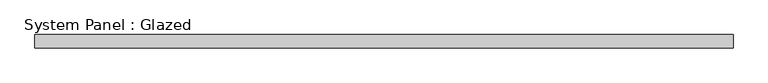
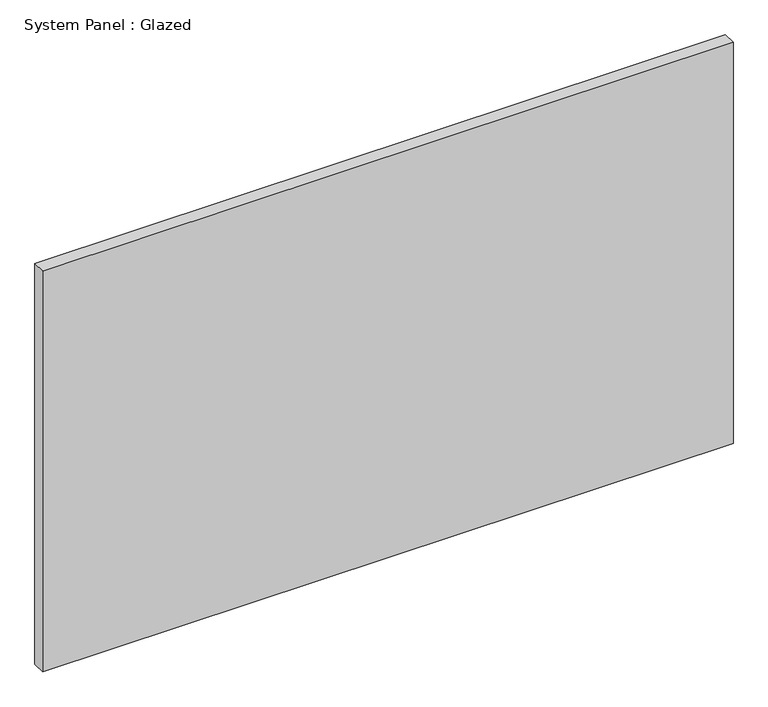
"""IFC4 building model written with IfcOpenShell, lengths in millimetres: plate geometry, System Panel : Glazed."""

from ifc_helpers import new_model, si_unit, origin, origin_with_axes, place, context, project, spatial, polyline, outline, extrude, source, transform, mapped, element, save


def system_panel_glazed_e21b380e(model_context):
    return source(origin(), model_context, "Body", "SweptSolid", [
        extrude(outline(polyline([(666.75, 19.05), (-666.75, 19.05), (-666.75, 44.45), (666.75, 44.45), (666.75, 19.05)])), origin_with_axes(), (0.0, 0.0, 1.0), 819.15),
    ])


if __name__ == "__main__":
    model = new_model("IFC4")
    model_context = context("Model", 3, world=origin())
    ifc_project = project(units=[si_unit("LENGTHUNIT", "METRE", prefix="MILLI")], contexts=[model_context])
    site = spatial("IfcSite", under=ifc_project)
    building = spatial("IfcBuilding", under=site)
    placement = place(None, origin())
    system_panel_glazed_shape = system_panel_glazed_e21b380e(model_context)
    element("IfcPlate", 1, ObjectType="System Panel : Glazed", at=placement, inside=building, context=model_context, shape_type="MappedRepresentation", body=[
        mapped(system_panel_glazed_shape, transform((0.0, 0.0, 0.0), x_axis=(1.0, 0.0, 0.0), y_axis=(0.0, 1.0, 0.0), z_axis=(0.0, 0.0, 1.0))),
    ])
    save(model, "model.ifc")

# Revit data of these elements
# Type "System Panel : Glazed"
#   Construction Type Id = "GSP4R"
#   Analytic Construction = "1/8 in Pilkington single glazing"
#   Visual Light Transmittance = 0.9
#   Solar Heat Gain Coefficient = 0.86
#   Heat Transfer Coefficient (U) = 1.18115 BTU/(h·ft²·°F)
# Element 1 (IfcPlate, "System Panel : Glazed")
#   Materials on its faces: "Glass"
# Materials
#   "Glass": class "Glass", colour RGB 0 128 192, transparency 0.75, Description = "Soda Lime Glass", Cost = 0
